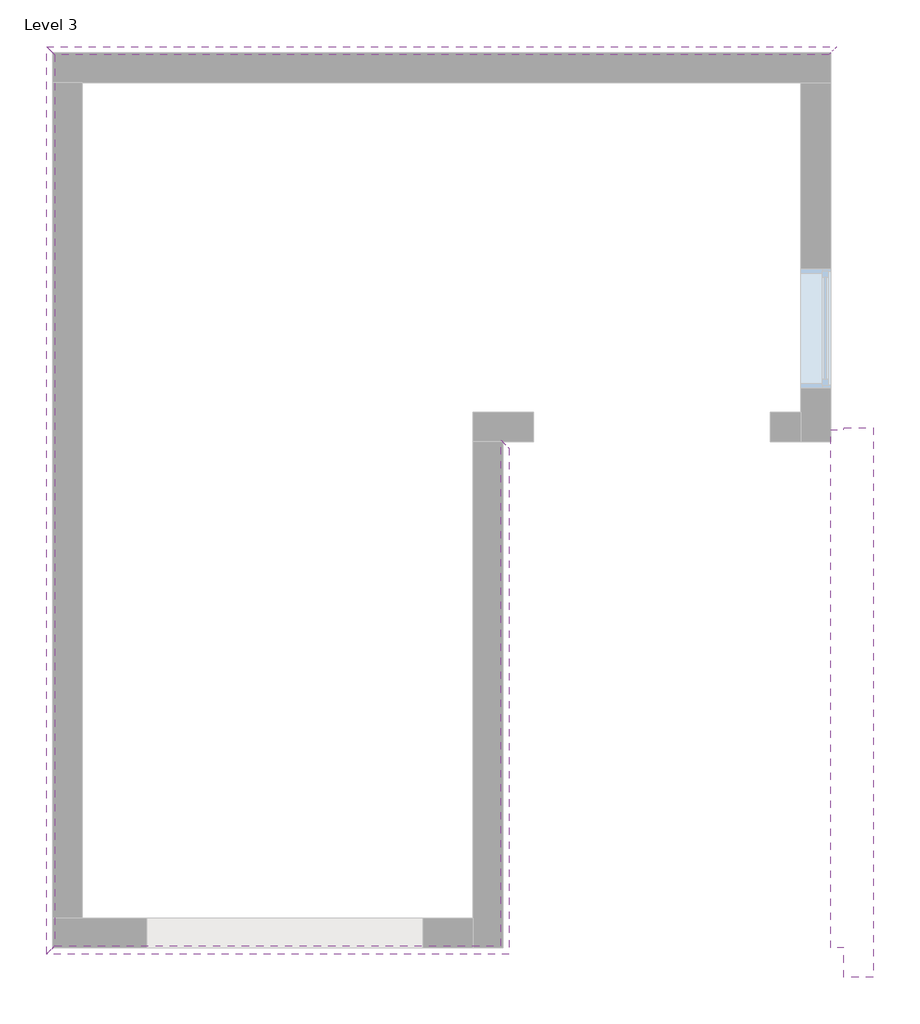
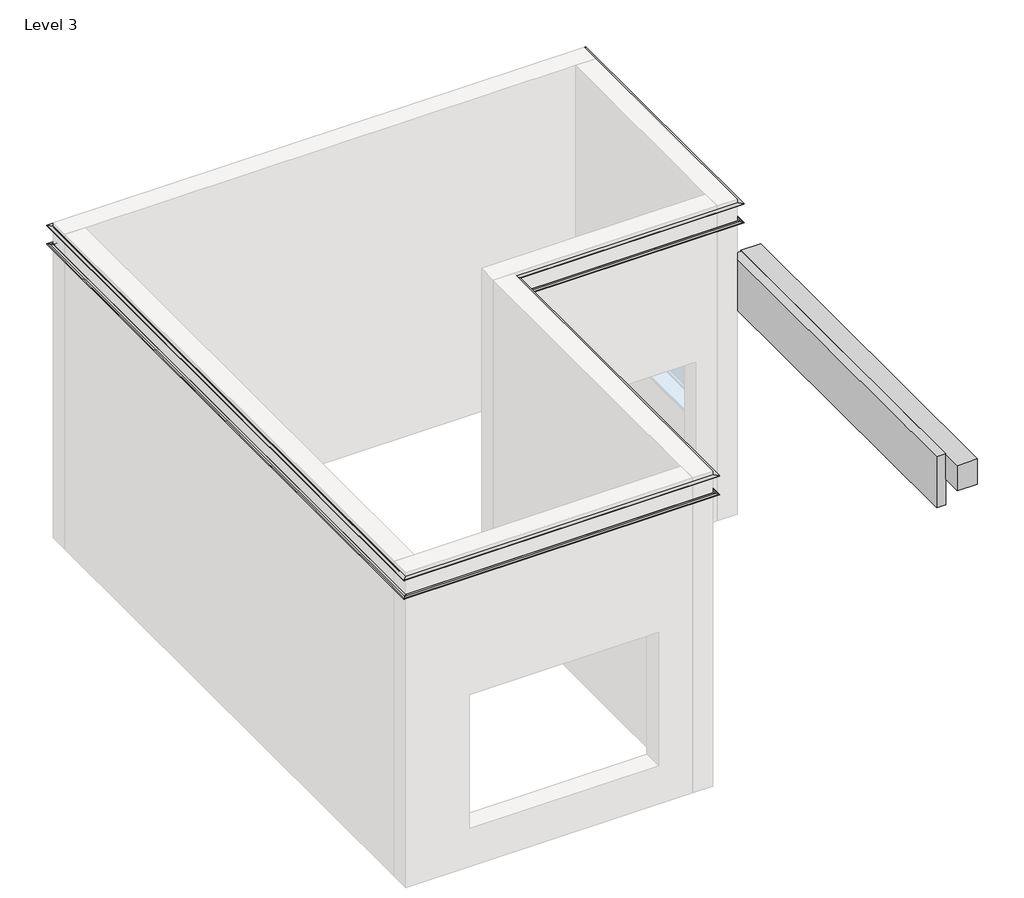
# One storey, part 2 of 2: 4 proxies.
"""IFC4 building model written with IfcOpenShell, lengths in millimetres."""

from ifc_helpers import new_model, si_unit, frame, origin, place, context, project, spatial, polyline, ellipse_curve, transform, mapped, element, save
from ifc_brep_helpers import plane_surface, cylinder_surface, revolved_surface, advanced_brep
from components import generic_models_3_generic_models_3_e8135b9d

model = new_model("IFC4")

# Units and contexts
model_context = context("Model", 3, world=origin())
ifc_project = project(units=[si_unit("LENGTHUNIT", "METRE", prefix="MILLI")], contexts=[model_context])

# Site, building, storey
site = spatial("IfcSite", under=ifc_project)
building = spatial("IfcBuilding", under=site)
storey = spatial("IfcBuildingStorey", under=building, Name="Level 3", Elevation=3200.4)

# Proxies
placement = place(None, origin())
element("IfcBuildingElementProxy", 1, Name="Cornice", ObjectType="Cornice", at=placement, inside=storey, context=model_context, shape_type="AdvancedBrep", body=[
    advanced_brep(
    [(-9818.4141584, 755.0106137, 6921.5), (-9755.1681584, 691.7646137, 6921.5), (-9755.1681584, 691.7646137, 6920.1203242), (-9759.5509676, 696.1474229, 6914.9465897), (-9783.1716584, 719.7681137, 6911.0098), (-9802.40954, 739.0059953, 6907.80348), (-9811.1751584, 747.7716137, 6897.456011), (-9811.1751584, 747.7716137, 6716.943989), (-9802.40954, 739.0059953, 6706.59652), (-9783.1716584, 719.7681137, 6703.3902), (-9759.5509676, 696.1474229, 6699.4534103), (-9755.1681584, 691.7646137, 6694.2796758), (-9755.1681584, 691.7646137, 6692.9), (-9818.4141584, 755.0106137, 6692.9), (-13260.1109834, 755.0106137, 6921.5), (-13260.1109834, 755.0106137, 6692.9), (-13323.3569834, 691.7646137, 6692.9), (-13323.3569834, 691.7646137, 6694.2796758), (-13318.9741742, 696.1474229, 6699.4534103), (-13295.3534834, 719.7681137, 6703.3902), (-13276.1156018, 739.0059953, 6706.59652), (-13267.3499834, 747.7716137, 6716.943989), (-13267.3499834, 747.7716137, 6897.456011), (-13276.1156018, 739.0059953, 6907.80348), (-13295.3534834, 719.7681137, 6911.0098), (-13318.9741742, 696.1474229, 6914.9465897), (-13323.3569834, 691.7646137, 6920.1203242), (-13323.3569834, 691.7646137, 6921.5)],
    [
        (0, 1),
        (1, 2),
        (2, 3, ellipse_curve(frame((-9760.4132584, 697.0097137, 6920.1203242), z_axis=(0.7071067811865493, 0.7071067811865458, 0.0), x_axis=(0.7071067811865456, -0.7071067811865493, 0.0)), 7.4176916, 5.2451)),
        (3, 4),
        (4, 5),
        (5, 6, ellipse_curve(frame((-9800.6849584, 737.2814137, 6897.456011), z_axis=(-0.7071067811865493, -0.7071067811865458, 0.0), x_axis=(-0.7071067811865456, 0.7071067811865493, 0.0)), 14.8353831, 10.4902)),
        (6, 7),
        (7, 8, ellipse_curve(frame((-9800.6849584, 737.2814137, 6716.943989), z_axis=(-0.7071067811865493, -0.7071067811865458, 0.0), x_axis=(-0.7071067811865456, 0.7071067811865493, 0.0)), 14.8353831, 10.4902)),
        (8, 9),
        (9, 10),
        (10, 11, ellipse_curve(frame((-9760.4132584, 697.0097137, 6694.2796758), z_axis=(0.7071067811865493, 0.7071067811865458, 0.0), x_axis=(0.7071067811865456, -0.7071067811865493, 0.0)), 7.4176916, 5.2451)),
        (11, 12),
        (12, 13),
        (13, 0),
        (14, 15),
        (15, 16),
        (16, 17),
        (17, 18, ellipse_curve(frame((-13318.1118834, 697.0097137, 6694.2796758), z_axis=(-0.7071067811865436, 0.7071067811865516, 0.0), x_axis=(0.7071067811865515, 0.7071067811865437, 0.0)), 7.4176916, 5.2451)),
        (18, 19),
        (19, 20),
        (20, 21, ellipse_curve(frame((-13277.8401834, 737.2814137, 6716.943989), z_axis=(0.7071067811865436, -0.7071067811865516, 0.0), x_axis=(-0.7071067811865515, -0.7071067811865437, 0.0)), 14.8353831, 10.4902)),
        (21, 22),
        (22, 23, ellipse_curve(frame((-13277.8401834, 737.2814137, 6897.456011), z_axis=(0.7071067811865436, -0.7071067811865516, 0.0), x_axis=(-0.7071067811865515, -0.7071067811865437, 0.0)), 14.8353831, 10.4902)),
        (23, 24),
        (24, 25),
        (25, 26, ellipse_curve(frame((-13318.1118834, 697.0097137, 6920.1203242), z_axis=(-0.7071067811865436, 0.7071067811865516, 0.0), x_axis=(0.7071067811865515, 0.7071067811865437, 0.0)), 7.4176916, 5.2451)),
        (26, 27),
        (27, 14),
        (0, 14),
        (27, 1),
        (26, 2),
        (25, 3),
        (24, 4),
        (23, 5),
        (22, 6),
        (21, 7),
        (20, 8),
        (19, 9),
        (18, 10),
        (17, 11),
        (16, 12),
        (15, 13),
    ],
    [
        plane_surface(frame((-9803.5297584, 740.1262137, 7112.0), z_axis=(0.7071067811865493, 0.7071067811865458, 0.0), x_axis=(-0.7071067811865458, 0.7071067811865493, 0.0))),
        plane_surface(frame((-13274.9953834, 740.1262137, 7112.0), z_axis=(-0.7071067811865436, 0.7071067811865516, 0.0), x_axis=(0.7071067811865516, 0.7071067811865436, 0.0))),
        plane_surface(frame((-9818.4141584, 755.0106137, 6921.5), z_axis=(0.0, 0.0, 1.0), x_axis=(-1.0, 0.0, 0.0))),
        plane_surface(frame((-9755.1681584, 691.7646137, 6921.5), z_axis=(0.0, -1.0, 0.0), x_axis=(-1.0, 0.0, 0.0))),
        cylinder_surface(frame((-9803.5297584, 697.0097137, 6920.1203242), z_axis=(1.0, 0.0, 0.0), x_axis=(0.0, -1.0, 0.0)), 5.2451),
        plane_surface(frame((-9759.5509676, 696.1474229, 6914.9465897), z_axis=(0.0, -0.16439930721687082, -0.9863938705135049), x_axis=(-1.0, 0.0, 0.0))),
        plane_surface(frame((-9783.1716584, 719.7681137, 6911.0098), z_axis=(0.0, -0.16439930721687146, -0.9863938705135048), x_axis=(-1.0, 0.0, 0.0))),
        revolved_surface(polyline([(-13288.33038339151, 726.7912137000001, 6897.456011), (-9790.194758408488, 726.7912137000001, 6897.456011)]), (-9803.5297584, 737.2814137, 6897.456011), (-1.0, 0.0, 0.0)),
        plane_surface(frame((-9811.1751584, 747.7716137, 6897.456011), z_axis=(0.0, -1.0, 0.0), x_axis=(-1.0, 0.0, 0.0))),
        revolved_surface(polyline([(-13288.33038339151, 726.7912137000001, 6716.943989), (-9790.194758408488, 726.7912137000001, 6716.943989)]), (-9803.5297584, 737.2814137, 6716.943989), (-1.0, 0.0, 0.0)),
        plane_surface(frame((-9802.40954, 739.0059953, 6706.59652), z_axis=(0.0, -0.1643993072168769, 0.9863938705135039), x_axis=(-1.0, 0.0, 0.0))),
        plane_surface(frame((-9783.1716584, 719.7681137, 6703.3902), z_axis=(0.0, -0.16439930721687793, 0.9863938705135037), x_axis=(-1.0, 0.0, 0.0))),
        cylinder_surface(frame((-9803.5297584, 697.0097137, 6694.2796758), z_axis=(1.0, 0.0, 0.0), x_axis=(0.0, -1.0, 0.0)), 5.2451),
        plane_surface(frame((-9755.1681584, 691.7646137, 6694.2796758), z_axis=(0.0, -1.0, 0.0), x_axis=(-1.0, 0.0, 0.0))),
        plane_surface(frame((-9755.1681584, 691.7646137, 6692.9), z_axis=(0.0, 0.0, -1.0), x_axis=(-1.0, 0.0, 0.0))),
        plane_surface(frame((-9818.4141584, 755.0106137, 6692.9), z_axis=(0.0, 1.0, 0.0), x_axis=(-1.0, 0.0, 0.0))),
    ],
    [
        (0, [[1, 2, 3, 4, 5, 6, 7, 8, 9, 10, 11, 12, 13, 14]]),
        (1, [[15, 16, 17, 18, 19, 20, 21, 22, 23, 24, 25, 26, 27, 28]]),
        (2, [[-1, 29, -28, 30]]),
        (3, [[-2, -30, -27, 31]]),
        (4, [[-3, -31, -26, 32]]),
        (5, [[-4, -32, -25, 33]]),
        (6, [[-5, -33, -24, 34]]),
        (7, [[-6, -34, -23, 35]]),
        (8, [[-7, -35, -22, 36]]),
        (9, [[-8, -36, -21, 37]]),
        (10, [[-9, -37, -20, 38]]),
        (11, [[-10, -38, -19, 39]]),
        (12, [[-11, -39, -18, 40]]),
        (13, [[-12, -40, -17, 41]]),
        (14, [[-13, -41, -16, 42]]),
        (15, [[-14, -42, -15, -29]]),
    ],
),
    advanced_brep(
    [(-9818.4141584, 4655.0020199, 6921.5), (-9755.1681584, 4591.7560199, 6921.5), (-9755.1681584, 4591.7560199, 6920.1203242), (-9759.5509676, 4596.1388291, 6914.9465897), (-9783.1716584, 4619.7595199, 6911.0098), (-9802.40954, 4638.9974015, 6907.80348), (-9811.1751584, 4647.7630199, 6897.456011), (-9811.1751584, 4647.7630199, 6716.943989), (-9802.40954, 4638.9974015, 6706.59652), (-9783.1716584, 4619.7595199, 6703.3902), (-9759.5509676, 4596.1388291, 6699.4534103), (-9755.1681584, 4591.7560199, 6694.2796758), (-9755.1681584, 4591.7560199, 6692.9), (-9818.4141584, 4655.0020199, 6692.9), (-9818.4141584, 755.0106137, 6921.5), (-9818.4141584, 755.0106137, 6692.9), (-9755.1681584, 691.7646137, 6692.9), (-9755.1681584, 691.7646137, 6694.2796758), (-9759.5509676, 696.1474229, 6699.4534103), (-9783.1716584, 719.7681137, 6703.3902), (-9802.40954, 739.0059953, 6706.59652), (-9811.1751584, 747.7716137, 6716.943989), (-9811.1751584, 747.7716137, 6897.456011), (-9802.40954, 739.0059953, 6907.80348), (-9783.1716584, 719.7681137, 6911.0098), (-9759.5509676, 696.1474229, 6914.9465897), (-9755.1681584, 691.7646137, 6920.1203242), (-9755.1681584, 691.7646137, 6921.5)],
    [
        (0, 1),
        (1, 2),
        (2, 3, ellipse_curve(frame((-9760.4132584, 4597.0011199, 6920.1203242), z_axis=(0.7071067811865493, 0.7071067811865458, 0.0), x_axis=(-0.7071067811865458, 0.7071067811865492, 0.0)), 7.4176916, 5.2451)),
        (3, 4),
        (4, 5),
        (5, 6, ellipse_curve(frame((-9800.6849584, 4637.2728199, 6897.456011), z_axis=(-0.7071067811865493, -0.7071067811865458, 0.0), x_axis=(0.7071067811865458, -0.7071067811865492, 0.0)), 14.8353831, 10.4902)),
        (6, 7),
        (7, 8, ellipse_curve(frame((-9800.6849584, 4637.2728199, 6716.943989), z_axis=(-0.7071067811865493, -0.7071067811865458, 0.0), x_axis=(0.7071067811865458, -0.7071067811865492, 0.0)), 14.8353831, 10.4902)),
        (8, 9),
        (9, 10),
        (10, 11, ellipse_curve(frame((-9760.4132584, 4597.0011199, 6694.2796758), z_axis=(0.7071067811865493, 0.7071067811865458, 0.0), x_axis=(-0.7071067811865458, 0.7071067811865492, 0.0)), 7.4176916, 5.2451)),
        (11, 12),
        (12, 13),
        (13, 0),
        (14, 15),
        (15, 16),
        (16, 17),
        (17, 18, ellipse_curve(frame((-9760.4132584, 697.0097137, 6694.2796758), z_axis=(-0.7071067811865493, -0.7071067811865458, 0.0), x_axis=(-0.7071067811865458, 0.7071067811865492, 0.0)), 7.4176916, 5.2451)),
        (18, 19),
        (19, 20),
        (20, 21, ellipse_curve(frame((-9800.6849584, 737.2814137, 6716.943989), z_axis=(0.7071067811865493, 0.7071067811865458, 0.0), x_axis=(0.7071067811865458, -0.7071067811865492, 0.0)), 14.8353831, 10.4902)),
        (21, 22),
        (22, 23, ellipse_curve(frame((-9800.6849584, 737.2814137, 6897.456011), z_axis=(0.7071067811865493, 0.7071067811865458, 0.0), x_axis=(0.7071067811865458, -0.7071067811865492, 0.0)), 14.8353831, 10.4902)),
        (23, 24),
        (24, 25),
        (25, 26, ellipse_curve(frame((-9760.4132584, 697.0097137, 6920.1203242), z_axis=(-0.7071067811865493, -0.7071067811865458, 0.0), x_axis=(-0.7071067811865458, 0.7071067811865492, 0.0)), 7.4176916, 5.2451)),
        (26, 27),
        (27, 14),
        (0, 14),
        (27, 1),
        (26, 2),
        (25, 3),
        (24, 4),
        (23, 5),
        (22, 6),
        (21, 7),
        (20, 8),
        (19, 9),
        (18, 10),
        (17, 11),
        (16, 12),
        (15, 13),
    ],
    [
        plane_surface(frame((-9803.5297584, 4640.1176199, 6502.4), z_axis=(0.7071067811865493, 0.7071067811865458, 0.0), x_axis=(0.7071067811865458, -0.7071067811865493, 0.0))),
        plane_surface(frame((-9803.5297584, 740.1262137, 7112.0), z_axis=(-0.7071067811865493, -0.7071067811865458, 0.0), x_axis=(-0.7071067811865458, 0.7071067811865493, 0.0))),
        plane_surface(frame((-9818.4141584, 4655.0020199, 6921.5), z_axis=(0.0, 0.0, 1.0), x_axis=(0.0, -1.0, 0.0))),
        plane_surface(frame((-9755.1681584, 4591.7560199, 6921.5), z_axis=(1.0, 0.0, 0.0), x_axis=(0.0, -1.0, 0.0))),
        cylinder_surface(frame((-9760.4132584, 4640.1176199, 6920.1203242), z_axis=(0.0, 1.0, 0.0), x_axis=(1.0, 0.0, 0.0)), 5.2451),
        plane_surface(frame((-9759.5509676, 4596.1388291, 6914.9465897), z_axis=(0.16439930721687082, 0.0, -0.9863938705135049), x_axis=(0.0, -1.0, 0.0))),
        plane_surface(frame((-9783.1716584, 4619.7595199, 6911.0098), z_axis=(0.16439930721687146, 0.0, -0.9863938705135048), x_axis=(0.0, -1.0, 0.0))),
        revolved_surface(polyline([(-9790.194758399999, 726.7912137084895, 6897.456011), (-9790.194758399999, 4647.7630199, 6897.456011)]), (-9800.6849584, 4640.1176199, 6897.456011), (0.0, -1.0, 0.0)),
        plane_surface(frame((-9811.1751584, 4647.7630199, 6897.456011), z_axis=(1.0, 0.0, 0.0), x_axis=(0.0, -1.0, 0.0))),
        revolved_surface(polyline([(-9790.194758399999, 726.7912137084895, 6716.943989), (-9790.194758399999, 4647.7630199, 6716.943989)]), (-9800.6849584, 4640.1176199, 6716.943989), (0.0, -1.0, 0.0)),
        plane_surface(frame((-9802.40954, 4638.9974015, 6706.59652), z_axis=(0.1643993072168769, 0.0, 0.9863938705135039), x_axis=(0.0, -1.0, 0.0))),
        plane_surface(frame((-9783.1716584, 4619.7595199, 6703.3902), z_axis=(0.16439930721687793, 0.0, 0.9863938705135037), x_axis=(0.0, -1.0, 0.0))),
        cylinder_surface(frame((-9760.4132584, 4640.1176199, 6694.2796758), z_axis=(0.0, 1.0, 0.0), x_axis=(1.0, 0.0, 0.0)), 5.2451),
        plane_surface(frame((-9755.1681584, 4591.7560199, 6694.2796758), z_axis=(1.0, 0.0, 0.0), x_axis=(0.0, -1.0, 0.0))),
        plane_surface(frame((-9755.1681584, 4591.7560199, 6692.9), z_axis=(0.0, 0.0, -1.0), x_axis=(0.0, -1.0, 0.0))),
        plane_surface(frame((-9818.4141584, 4655.0020199, 6692.9), z_axis=(-1.0, 0.0, 0.0), x_axis=(0.0, -1.0, 0.0))),
    ],
    [
        (0, [[1, 2, 3, 4, 5, 6, 7, 8, 9, 10, 11, 12, 13, 14]]),
        (1, [[15, 16, 17, 18, 19, 20, 21, 22, 23, 24, 25, 26, 27, 28]]),
        (2, [[-1, 29, -28, 30]]),
        (3, [[-2, -30, -27, 31]]),
        (4, [[-3, -31, -26, 32]]),
        (5, [[-4, -32, -25, 33]]),
        (6, [[-5, -33, -24, 34]]),
        (7, [[-6, -34, -23, 35]]),
        (8, [[-7, -35, -22, 36]]),
        (9, [[-8, -36, -21, 37]]),
        (10, [[-9, -37, -20, 38]]),
        (11, [[-10, -38, -19, 39]]),
        (12, [[-11, -39, -18, 40]]),
        (13, [[-12, -40, -17, 41]]),
        (14, [[-13, -41, -16, 42]]),
        (15, [[-14, -42, -15, -29]]),
    ],
),
])
element("IfcBuildingElementProxy", 2, Name="Cornice", ObjectType="Cornice", at=placement, inside=storey, context=model_context, shape_type="AdvancedBrep", body=[
    advanced_brep(
    [(-7289.8797834, 4655.0020199, 6921.5), (-7226.6337834, 4591.7560199, 6921.5), (-7226.6337834, 4591.7560199, 6920.1203242), (-7231.0165926, 4596.1388291, 6914.9465897), (-7254.6372834, 4619.7595199, 6911.0098), (-7273.875165, 4638.9974015, 6907.80348), (-7282.6407834, 4647.7630199, 6897.456011), (-7282.6407834, 4647.7630199, 6716.943989), (-7273.875165, 4638.9974015, 6706.59652), (-7254.6372834, 4619.7595199, 6703.3902), (-7231.0165926, 4596.1388291, 6699.4534103), (-7226.6337834, 4591.7560199, 6694.2796758), (-7226.6337834, 4591.7560199, 6692.9), (-7289.8797834, 4655.0020199, 6692.9), (-9818.4141584, 4655.0020199, 6921.5), (-9818.4141584, 4655.0020199, 6692.9), (-9755.1681584, 4591.7560199, 6692.9), (-9755.1681584, 4591.7560199, 6694.2796758), (-9759.5509676, 4596.1388291, 6699.4534103), (-9783.1716584, 4619.7595199, 6703.3902), (-9802.40954, 4638.9974015, 6706.59652), (-9811.1751584, 4647.7630199, 6716.943989), (-9811.1751584, 4647.7630199, 6897.456011), (-9802.40954, 4638.9974015, 6907.80348), (-9783.1716584, 4619.7595199, 6911.0098), (-9759.5509676, 4596.1388291, 6914.9465897), (-9755.1681584, 4591.7560199, 6920.1203242), (-9755.1681584, 4591.7560199, 6921.5)],
    [
        (0, 1),
        (1, 2),
        (2, 3, ellipse_curve(frame((-7231.8788834, 4597.0011199, 6920.1203242), z_axis=(0.707106781186552, 0.7071067811865431, 0.0), x_axis=(0.7071067811865431, -0.707106781186552, 0.0)), 7.4176916, 5.2451)),
        (3, 4),
        (4, 5),
        (5, 6, ellipse_curve(frame((-7272.1505834, 4637.2728199, 6897.456011), z_axis=(-0.707106781186552, -0.7071067811865431, 0.0), x_axis=(-0.7071067811865431, 0.707106781186552, 0.0)), 14.8353831, 10.4902)),
        (6, 7),
        (7, 8, ellipse_curve(frame((-7272.1505834, 4637.2728199, 6716.943989), z_axis=(-0.707106781186552, -0.7071067811865431, 0.0), x_axis=(-0.7071067811865431, 0.707106781186552, 0.0)), 14.8353831, 10.4902)),
        (8, 9),
        (9, 10),
        (10, 11, ellipse_curve(frame((-7231.8788834, 4597.0011199, 6694.2796758), z_axis=(0.707106781186552, 0.7071067811865431, 0.0), x_axis=(0.7071067811865431, -0.707106781186552, 0.0)), 7.4176916, 5.2451)),
        (11, 12),
        (12, 13),
        (13, 0),
        (14, 15),
        (15, 16),
        (16, 17),
        (17, 18, ellipse_curve(frame((-9760.4132584, 4597.0011199, 6694.2796758), z_axis=(-0.7071067811865493, -0.7071067811865458, 0.0), x_axis=(0.7071067811865458, -0.7071067811865493, 0.0)), 7.4176916, 5.2451)),
        (18, 19),
        (19, 20),
        (20, 21, ellipse_curve(frame((-9800.6849584, 4637.2728199, 6716.943989), z_axis=(0.7071067811865493, 0.7071067811865458, 0.0), x_axis=(-0.7071067811865458, 0.7071067811865493, 0.0)), 14.8353831, 10.4902)),
        (21, 22),
        (22, 23, ellipse_curve(frame((-9800.6849584, 4637.2728199, 6897.456011), z_axis=(0.7071067811865493, 0.7071067811865458, 0.0), x_axis=(-0.7071067811865458, 0.7071067811865493, 0.0)), 14.8353831, 10.4902)),
        (23, 24),
        (24, 25),
        (25, 26, ellipse_curve(frame((-9760.4132584, 4597.0011199, 6920.1203242), z_axis=(-0.7071067811865493, -0.7071067811865458, 0.0), x_axis=(0.7071067811865458, -0.7071067811865493, 0.0)), 7.4176916, 5.2451)),
        (26, 27),
        (27, 14),
        (0, 14),
        (27, 1),
        (26, 2),
        (25, 3),
        (24, 4),
        (23, 5),
        (22, 6),
        (21, 7),
        (20, 8),
        (19, 9),
        (18, 10),
        (17, 11),
        (16, 12),
        (15, 13),
    ],
    [
        plane_surface(frame((-7274.9953834, 4640.1176199, 7112.0), z_axis=(0.707106781186552, 0.7071067811865431, 0.0), x_axis=(-0.7071067811865431, 0.707106781186552, 0.0))),
        plane_surface(frame((-9803.5297584, 4640.1176199, 6502.4), z_axis=(-0.7071067811865493, -0.7071067811865458, 0.0), x_axis=(0.7071067811865458, -0.7071067811865493, 0.0))),
        plane_surface(frame((-7289.8797834, 4655.0020199, 6921.5), z_axis=(0.0, 0.0, 1.0), x_axis=(-1.0, 0.0, 0.0))),
        plane_surface(frame((-7226.6337834, 4591.7560199, 6921.5), z_axis=(0.0, -1.0, 0.0), x_axis=(-1.0, 0.0, 0.0))),
        cylinder_surface(frame((-7274.9953834, 4597.0011199, 6920.1203242), z_axis=(1.0, 0.0, 0.0), x_axis=(0.0, -1.0, 0.0)), 5.2451),
        plane_surface(frame((-7231.0165926, 4596.1388291, 6914.9465897), z_axis=(0.0, -0.16439930721687082, -0.9863938705135049), x_axis=(-1.0, 0.0, 0.0))),
        plane_surface(frame((-7254.6372834, 4619.7595199, 6911.0098), z_axis=(0.0, -0.16439930721687146, -0.9863938705135048), x_axis=(-1.0, 0.0, 0.0))),
        revolved_surface(polyline([(-9811.1751584, 4626.7826199, 6897.456011), (-7261.66038340849, 4626.7826199, 6897.456011)]), (-7274.9953834, 4637.2728199, 6897.456011), (-1.0, 0.0, 0.0)),
        plane_surface(frame((-7282.6407834, 4647.7630199, 6897.456011), z_axis=(0.0, -1.0, 0.0), x_axis=(-1.0, 0.0, 0.0))),
        revolved_surface(polyline([(-9811.1751584, 4626.7826199, 6716.943989), (-7261.66038340849, 4626.7826199, 6716.943989)]), (-7274.9953834, 4637.2728199, 6716.943989), (-1.0, 0.0, 0.0)),
        plane_surface(frame((-7273.875165, 4638.9974015, 6706.59652), z_axis=(0.0, -0.1643993072168769, 0.9863938705135039), x_axis=(-1.0, 0.0, 0.0))),
        plane_surface(frame((-7254.6372834, 4619.7595199, 6703.3902), z_axis=(0.0, -0.16439930721687793, 0.9863938705135037), x_axis=(-1.0, 0.0, 0.0))),
        cylinder_surface(frame((-7274.9953834, 4597.0011199, 6694.2796758), z_axis=(1.0, 0.0, 0.0), x_axis=(0.0, -1.0, 0.0)), 5.2451),
        plane_surface(frame((-7226.6337834, 4591.7560199, 6694.2796758), z_axis=(0.0, -1.0, 0.0), x_axis=(-1.0, 0.0, 0.0))),
        plane_surface(frame((-7226.6337834, 4591.7560199, 6692.9), z_axis=(0.0, 0.0, -1.0), x_axis=(-1.0, 0.0, 0.0))),
        plane_surface(frame((-7289.8797834, 4655.0020199, 6692.9), z_axis=(0.0, 1.0, 0.0), x_axis=(-1.0, 0.0, 0.0))),
    ],
    [
        (0, [[1, 2, 3, 4, 5, 6, 7, 8, 9, 10, 11, 12, 13, 14]]),
        (1, [[15, 16, 17, 18, 19, 20, 21, 22, 23, 24, 25, 26, 27, 28]]),
        (2, [[-1, 29, -28, 30]]),
        (3, [[-2, -30, -27, 31]]),
        (4, [[-3, -31, -26, 32]]),
        (5, [[-4, -32, -25, 33]]),
        (6, [[-5, -33, -24, 34]]),
        (7, [[-6, -34, -23, 35]]),
        (8, [[-7, -35, -22, 36]]),
        (9, [[-8, -36, -21, 37]]),
        (10, [[-9, -37, -20, 38]]),
        (11, [[-10, -38, -19, 39]]),
        (12, [[-11, -39, -18, 40]]),
        (13, [[-12, -40, -17, 41]]),
        (14, [[-13, -41, -16, 42]]),
        (15, [[-14, -42, -15, -29]]),
    ],
),
    advanced_brep(
    [(-7289.8797834, 7625.2418137, 6921.5), (-7226.6337834, 7688.4878137, 6921.5), (-7226.6337834, 7688.4878137, 6920.1203242), (-7231.0165926, 7684.1050045, 6914.9465897), (-7254.6372834, 7660.4843137, 6911.0098), (-7273.875165, 7641.2464321, 6907.80348), (-7282.6407834, 7632.4808137, 6897.456011), (-7282.6407834, 7632.4808137, 6716.943989), (-7273.875165, 7641.2464321, 6706.59652), (-7254.6372834, 7660.4843137, 6703.3902), (-7231.0165926, 7684.1050045, 6699.4534103), (-7226.6337834, 7688.4878137, 6694.2796758), (-7226.6337834, 7688.4878137, 6692.9), (-7289.8797834, 7625.2418137, 6692.9), (-7289.8797834, 4655.0020199, 6921.5), (-7289.8797834, 4655.0020199, 6692.9), (-7226.6337834, 4591.7560199, 6692.9), (-7226.6337834, 4591.7560199, 6694.2796758), (-7231.0165926, 4596.1388291, 6699.4534103), (-7254.6372834, 4619.7595199, 6703.3902), (-7273.875165, 4638.9974015, 6706.59652), (-7282.6407834, 4647.7630199, 6716.943989), (-7282.6407834, 4647.7630199, 6897.456011), (-7273.875165, 4638.9974015, 6907.80348), (-7254.6372834, 4619.7595199, 6911.0098), (-7231.0165926, 4596.1388291, 6914.9465897), (-7226.6337834, 4591.7560199, 6920.1203242), (-7226.6337834, 4591.7560199, 6921.5)],
    [
        (0, 1),
        (1, 2),
        (2, 3, ellipse_curve(frame((-7231.8788834, 7683.2427137, 6920.1203242), z_axis=(-0.7071067811865458, 0.7071067811865493, 0.0), x_axis=(0.7071067811865493, 0.7071067811865456, 0.0)), 7.4176916, 5.2451)),
        (3, 4),
        (4, 5),
        (5, 6, ellipse_curve(frame((-7272.1505834, 7642.9710137, 6897.456011), z_axis=(0.7071067811865458, -0.7071067811865493, 0.0), x_axis=(-0.7071067811865493, -0.7071067811865456, 0.0)), 14.8353831, 10.4902)),
        (6, 7),
        (7, 8, ellipse_curve(frame((-7272.1505834, 7642.9710137, 6716.943989), z_axis=(0.7071067811865458, -0.7071067811865493, 0.0), x_axis=(-0.7071067811865493, -0.7071067811865456, 0.0)), 14.8353831, 10.4902)),
        (8, 9),
        (9, 10),
        (10, 11, ellipse_curve(frame((-7231.8788834, 7683.2427137, 6694.2796758), z_axis=(-0.7071067811865458, 0.7071067811865493, 0.0), x_axis=(0.7071067811865493, 0.7071067811865456, 0.0)), 7.4176916, 5.2451)),
        (11, 12),
        (12, 13),
        (13, 0),
        (14, 15),
        (15, 16),
        (16, 17),
        (17, 18, ellipse_curve(frame((-7231.8788834, 4597.0011199, 6694.2796758), z_axis=(-0.707106781186552, -0.7071067811865431, 0.0), x_axis=(-0.7071067811865432, 0.7071067811865518, 0.0)), 7.4176916, 5.2451)),
        (18, 19),
        (19, 20),
        (20, 21, ellipse_curve(frame((-7272.1505834, 4637.2728199, 6716.943989), z_axis=(0.707106781186552, 0.7071067811865431, 0.0), x_axis=(0.7071067811865432, -0.7071067811865518, 0.0)), 14.8353831, 10.4902)),
        (21, 22),
        (22, 23, ellipse_curve(frame((-7272.1505834, 4637.2728199, 6897.456011), z_axis=(0.707106781186552, 0.7071067811865431, 0.0), x_axis=(0.7071067811865432, -0.7071067811865518, 0.0)), 14.8353831, 10.4902)),
        (23, 24),
        (24, 25),
        (25, 26, ellipse_curve(frame((-7231.8788834, 4597.0011199, 6920.1203242), z_axis=(-0.707106781186552, -0.7071067811865431, 0.0), x_axis=(-0.7071067811865432, 0.7071067811865518, 0.0)), 7.4176916, 5.2451)),
        (26, 27),
        (27, 14),
        (0, 14),
        (27, 1),
        (26, 2),
        (25, 3),
        (24, 4),
        (23, 5),
        (22, 6),
        (21, 7),
        (20, 8),
        (19, 9),
        (18, 10),
        (17, 11),
        (16, 12),
        (15, 13),
    ],
    [
        plane_surface(frame((-7274.9953834, 7640.1262137, 7112.0), z_axis=(-0.7071067811865458, 0.7071067811865493, 0.0), x_axis=(-0.7071067811865493, -0.7071067811865458, 0.0))),
        plane_surface(frame((-7274.9953834, 4640.1176199, 7112.0), z_axis=(-0.707106781186552, -0.7071067811865431, 0.0), x_axis=(-0.7071067811865431, 0.707106781186552, 0.0))),
        plane_surface(frame((-7289.8797834, 7625.2418137, 6921.5), z_axis=(0.0, 0.0, 1.0), x_axis=(0.0, -1.0, 0.0))),
        plane_surface(frame((-7226.6337834, 7688.4878137, 6921.5), z_axis=(1.0, 0.0, 0.0), x_axis=(0.0, -1.0, 0.0))),
        cylinder_surface(frame((-7231.8788834, 7640.1262137, 6920.1203242), z_axis=(0.0, 1.0, 0.0), x_axis=(1.0, 0.0, 0.0)), 5.2451),
        plane_surface(frame((-7231.0165926, 7684.1050045, 6914.9465897), z_axis=(0.16439930721687082, 0.0, -0.9863938705135049), x_axis=(0.0, -1.0, 0.0))),
        plane_surface(frame((-7254.6372834, 7660.4843137, 6911.0098), z_axis=(0.16439930721687146, 0.0, -0.9863938705135048), x_axis=(0.0, -1.0, 0.0))),
        revolved_surface(polyline([(-7261.6603834, 4626.78261990849, 6897.456011), (-7261.6603834, 7653.46121369151, 6897.456011)]), (-7272.1505834, 7640.1262137, 6897.456011), (0.0, -1.0, 0.0)),
        plane_surface(frame((-7282.6407834, 7632.4808137, 6897.456011), z_axis=(1.0, 0.0, 0.0), x_axis=(0.0, -1.0, 0.0))),
        revolved_surface(polyline([(-7261.6603834, 4626.78261990849, 6716.943989), (-7261.6603834, 7653.46121369151, 6716.943989)]), (-7272.1505834, 7640.1262137, 6716.943989), (0.0, -1.0, 0.0)),
        plane_surface(frame((-7273.875165, 7641.2464321, 6706.59652), z_axis=(0.1643993072168769, 0.0, 0.9863938705135039), x_axis=(0.0, -1.0, 0.0))),
        plane_surface(frame((-7254.6372834, 7660.4843137, 6703.3902), z_axis=(0.16439930721687793, 0.0, 0.9863938705135037), x_axis=(0.0, -1.0, 0.0))),
        cylinder_surface(frame((-7231.8788834, 7640.1262137, 6694.2796758), z_axis=(0.0, 1.0, 0.0), x_axis=(1.0, 0.0, 0.0)), 5.2451),
        plane_surface(frame((-7226.6337834, 7688.4878137, 6694.2796758), z_axis=(1.0, 0.0, 0.0), x_axis=(0.0, -1.0, 0.0))),
        plane_surface(frame((-7226.6337834, 7688.4878137, 6692.9), z_axis=(0.0, 0.0, -1.0), x_axis=(0.0, -1.0, 0.0))),
        plane_surface(frame((-7289.8797834, 7625.2418137, 6692.9), z_axis=(-1.0, 0.0, 0.0), x_axis=(0.0, -1.0, 0.0))),
    ],
    [
        (0, [[1, 2, 3, 4, 5, 6, 7, 8, 9, 10, 11, 12, 13, 14]]),
        (1, [[15, 16, 17, 18, 19, 20, 21, 22, 23, 24, 25, 26, 27, 28]]),
        (2, [[-1, 29, -28, 30]]),
        (3, [[-2, -30, -27, 31]]),
        (4, [[-3, -31, -26, 32]]),
        (5, [[-4, -32, -25, 33]]),
        (6, [[-5, -33, -24, 34]]),
        (7, [[-6, -34, -23, 35]]),
        (8, [[-7, -35, -22, 36]]),
        (9, [[-8, -36, -21, 37]]),
        (10, [[-9, -37, -20, 38]]),
        (11, [[-10, -38, -19, 39]]),
        (12, [[-11, -39, -18, 40]]),
        (13, [[-12, -40, -17, 41]]),
        (14, [[-13, -41, -16, 42]]),
        (15, [[-14, -42, -15, -29]]),
    ],
),
    advanced_brep(
    [(-13260.1109834, 755.0106137, 6921.5), (-13323.3569834, 691.7646137, 6921.5), (-13323.3569834, 691.7646137, 6920.1203242), (-13318.9741742, 696.1474229, 6914.9465897), (-13295.3534834, 719.7681137, 6911.0098), (-13276.1156018, 739.0059953, 6907.80348), (-13267.3499834, 747.7716137, 6897.456011), (-13267.3499834, 747.7716137, 6716.943989), (-13276.1156018, 739.0059953, 6706.59652), (-13295.3534834, 719.7681137, 6703.3902), (-13318.9741742, 696.1474229, 6699.4534103), (-13323.3569834, 691.7646137, 6694.2796758), (-13323.3569834, 691.7646137, 6692.9), (-13260.1109834, 755.0106137, 6692.9), (-13260.1109834, 7625.2418137, 6921.5), (-13260.1109834, 7625.2418137, 6692.9), (-13323.3569834, 7688.4878137, 6692.9), (-13323.3569834, 7688.4878137, 6694.2796758), (-13318.9741742, 7684.1050045, 6699.4534103), (-13295.3534834, 7660.4843137, 6703.3902), (-13276.1156018, 7641.2464321, 6706.59652), (-13267.3499834, 7632.4808137, 6716.943989), (-13267.3499834, 7632.4808137, 6897.456011), (-13276.1156018, 7641.2464321, 6907.80348), (-13295.3534834, 7660.4843137, 6911.0098), (-13318.9741742, 7684.1050045, 6914.9465897), (-13323.3569834, 7688.4878137, 6920.1203242), (-13323.3569834, 7688.4878137, 6921.5)],
    [
        (0, 1),
        (1, 2),
        (2, 3, ellipse_curve(frame((-13318.1118834, 697.0097137, 6920.1203242), z_axis=(0.7071067811865436, -0.7071067811865516, 0.0), x_axis=(-0.7071067811865516, -0.7071067811865435, 0.0)), 7.4176916, 5.2451)),
        (3, 4),
        (4, 5),
        (5, 6, ellipse_curve(frame((-13277.8401834, 737.2814137, 6897.456011), z_axis=(-0.7071067811865436, 0.7071067811865516, 0.0), x_axis=(0.7071067811865516, 0.7071067811865435, 0.0)), 14.8353831, 10.4902)),
        (6, 7),
        (7, 8, ellipse_curve(frame((-13277.8401834, 737.2814137, 6716.943989), z_axis=(-0.7071067811865436, 0.7071067811865516, 0.0), x_axis=(0.7071067811865516, 0.7071067811865435, 0.0)), 14.8353831, 10.4902)),
        (8, 9),
        (9, 10),
        (10, 11, ellipse_curve(frame((-13318.1118834, 697.0097137, 6694.2796758), z_axis=(0.7071067811865436, -0.7071067811865516, 0.0), x_axis=(-0.7071067811865516, -0.7071067811865435, 0.0)), 7.4176916, 5.2451)),
        (11, 12),
        (12, 13),
        (13, 0),
        (14, 15),
        (15, 16),
        (16, 17),
        (17, 18, ellipse_curve(frame((-13318.1118834, 7683.2427137, 6694.2796758), z_axis=(0.7071067811865493, 0.7071067811865458, 0.0), x_axis=(0.7071067811865459, -0.7071067811865492, 0.0)), 7.4176916, 5.2451)),
        (18, 19),
        (19, 20),
        (20, 21, ellipse_curve(frame((-13277.8401834, 7642.9710137, 6716.943989), z_axis=(-0.7071067811865493, -0.7071067811865458, 0.0), x_axis=(-0.7071067811865459, 0.7071067811865492, 0.0)), 14.8353831, 10.4902)),
        (21, 22),
        (22, 23, ellipse_curve(frame((-13277.8401834, 7642.9710137, 6897.456011), z_axis=(-0.7071067811865493, -0.7071067811865458, 0.0), x_axis=(-0.7071067811865459, 0.7071067811865492, 0.0)), 14.8353831, 10.4902)),
        (23, 24),
        (24, 25),
        (25, 26, ellipse_curve(frame((-13318.1118834, 7683.2427137, 6920.1203242), z_axis=(0.7071067811865493, 0.7071067811865458, 0.0), x_axis=(0.7071067811865459, -0.7071067811865492, 0.0)), 7.4176916, 5.2451)),
        (26, 27),
        (27, 14),
        (0, 14),
        (27, 1),
        (26, 2),
        (25, 3),
        (24, 4),
        (23, 5),
        (22, 6),
        (21, 7),
        (20, 8),
        (19, 9),
        (18, 10),
        (17, 11),
        (16, 12),
        (15, 13),
    ],
    [
        plane_surface(frame((-13274.9953834, 740.1262137, 7112.0), z_axis=(0.7071067811865436, -0.7071067811865516, 0.0), x_axis=(0.7071067811865516, 0.7071067811865436, 0.0))),
        plane_surface(frame((-13274.9953834, 7640.1262137, 7112.0), z_axis=(0.7071067811865493, 0.7071067811865458, 0.0), x_axis=(0.7071067811865458, -0.7071067811865493, 0.0))),
        plane_surface(frame((-13260.1109834, 755.0106137, 6921.5), z_axis=(0.0, 0.0, 1.0), x_axis=(0.0, 1.0, 0.0))),
        plane_surface(frame((-13323.3569834, 691.7646137, 6921.5), z_axis=(-1.0, 0.0, 0.0), x_axis=(0.0, 1.0, 0.0))),
        cylinder_surface(frame((-13318.1118834, 740.1262137, 6920.1203242), z_axis=(0.0, -1.0, 0.0), x_axis=(-1.0, 0.0, 0.0)), 5.2451),
        plane_surface(frame((-13318.9741742, 696.1474229, 6914.9465897), z_axis=(-0.16439930721687082, 0.0, -0.9863938705135049), x_axis=(0.0, 1.0, 0.0))),
        plane_surface(frame((-13295.3534834, 719.7681137, 6911.0098), z_axis=(-0.16439930721687146, 0.0, -0.9863938705135048), x_axis=(0.0, 1.0, 0.0))),
        revolved_surface(polyline([(-13288.3303834, 7653.46121369151, 6897.456011), (-13288.3303834, 726.7912137084897, 6897.456011)]), (-13277.8401834, 740.1262137, 6897.456011), (0.0, 1.0, 0.0)),
        plane_surface(frame((-13267.3499834, 747.7716137, 6897.456011), z_axis=(-1.0, 0.0, 0.0), x_axis=(0.0, 1.0, 0.0))),
        revolved_surface(polyline([(-13288.3303834, 7653.46121369151, 6716.943989), (-13288.3303834, 726.7912137084897, 6716.943989)]), (-13277.8401834, 740.1262137, 6716.943989), (0.0, 1.0, 0.0)),
        plane_surface(frame((-13276.1156018, 739.0059953, 6706.59652), z_axis=(-0.1643993072168769, 0.0, 0.9863938705135039), x_axis=(0.0, 1.0, 0.0))),
        plane_surface(frame((-13295.3534834, 719.7681137, 6703.3902), z_axis=(-0.16439930721687793, 0.0, 0.9863938705135037), x_axis=(0.0, 1.0, 0.0))),
        cylinder_surface(frame((-13318.1118834, 740.1262137, 6694.2796758), z_axis=(0.0, -1.0, 0.0), x_axis=(-1.0, 0.0, 0.0)), 5.2451),
        plane_surface(frame((-13323.3569834, 691.7646137, 6694.2796758), z_axis=(-1.0, 0.0, 0.0), x_axis=(0.0, 1.0, 0.0))),
        plane_surface(frame((-13323.3569834, 691.7646137, 6692.9), z_axis=(0.0, 0.0, -1.0), x_axis=(0.0, 1.0, 0.0))),
        plane_surface(frame((-13260.1109834, 755.0106137, 6692.9), z_axis=(1.0, 0.0, 0.0), x_axis=(0.0, 1.0, 0.0))),
    ],
    [
        (0, [[1, 2, 3, 4, 5, 6, 7, 8, 9, 10, 11, 12, 13, 14]]),
        (1, [[15, 16, 17, 18, 19, 20, 21, 22, 23, 24, 25, 26, 27, 28]]),
        (2, [[-1, 29, -28, 30]]),
        (3, [[-2, -30, -27, 31]]),
        (4, [[-3, -31, -26, 32]]),
        (5, [[-4, -32, -25, 33]]),
        (6, [[-5, -33, -24, 34]]),
        (7, [[-6, -34, -23, 35]]),
        (8, [[-7, -35, -22, 36]]),
        (9, [[-8, -36, -21, 37]]),
        (10, [[-9, -37, -20, 38]]),
        (11, [[-10, -38, -19, 39]]),
        (12, [[-11, -39, -18, 40]]),
        (13, [[-12, -40, -17, 41]]),
        (14, [[-13, -41, -16, 42]]),
        (15, [[-14, -42, -15, -29]]),
    ],
),
])
element("IfcBuildingElementProxy", 3, Name="Cornice", ObjectType="Cornice", at=placement, inside=storey, context=model_context, shape_type="AdvancedBrep", body=[
    advanced_brep(
    [(-13260.1109834, 7625.2418137, 6921.5), (-13323.3569834, 7688.4878137, 6921.5), (-13323.3569834, 7688.4878137, 6920.1203242), (-13318.9741742, 7684.1050045, 6914.9465897), (-13295.3534834, 7660.4843137, 6911.0098), (-13276.1156018, 7641.2464321, 6907.80348), (-13267.3499834, 7632.4808137, 6897.456011), (-13267.3499834, 7632.4808137, 6716.943989), (-13276.1156018, 7641.2464321, 6706.59652), (-13295.3534834, 7660.4843137, 6703.3902), (-13318.9741742, 7684.1050045, 6699.4534103), (-13323.3569834, 7688.4878137, 6694.2796758), (-13323.3569834, 7688.4878137, 6692.9), (-13260.1109834, 7625.2418137, 6692.9), (-7289.8797834, 7625.2418137, 6921.5), (-7289.8797834, 7625.2418137, 6692.9), (-7226.6337834, 7688.4878137, 6692.9), (-7226.6337834, 7688.4878137, 6694.2796758), (-7231.0165926, 7684.1050045, 6699.4534103), (-7254.6372834, 7660.4843137, 6703.3902), (-7273.875165, 7641.2464321, 6706.59652), (-7282.6407834, 7632.4808137, 6716.943989), (-7282.6407834, 7632.4808137, 6897.456011), (-7273.875165, 7641.2464321, 6907.80348), (-7254.6372834, 7660.4843137, 6911.0098), (-7231.0165926, 7684.1050045, 6914.9465897), (-7226.6337834, 7688.4878137, 6920.1203242), (-7226.6337834, 7688.4878137, 6921.5)],
    [
        (0, 1),
        (1, 2),
        (2, 3, ellipse_curve(frame((-13318.1118834, 7683.2427137, 6920.1203242), z_axis=(-0.7071067811865493, -0.7071067811865458, 0.0), x_axis=(-0.7071067811865457, 0.7071067811865492, 0.0)), 7.4176916, 5.2451)),
        (3, 4),
        (4, 5),
        (5, 6, ellipse_curve(frame((-13277.8401834, 7642.9710137, 6897.456011), z_axis=(0.7071067811865493, 0.7071067811865458, 0.0), x_axis=(0.7071067811865457, -0.7071067811865492, 0.0)), 14.8353831, 10.4902)),
        (6, 7),
        (7, 8, ellipse_curve(frame((-13277.8401834, 7642.9710137, 6716.943989), z_axis=(0.7071067811865493, 0.7071067811865458, 0.0), x_axis=(0.7071067811865457, -0.7071067811865492, 0.0)), 14.8353831, 10.4902)),
        (8, 9),
        (9, 10),
        (10, 11, ellipse_curve(frame((-13318.1118834, 7683.2427137, 6694.2796758), z_axis=(-0.7071067811865493, -0.7071067811865458, 0.0), x_axis=(-0.7071067811865457, 0.7071067811865492, 0.0)), 7.4176916, 5.2451)),
        (11, 12),
        (12, 13),
        (13, 0),
        (14, 15),
        (15, 16),
        (16, 17),
        (17, 18, ellipse_curve(frame((-7231.8788834, 7683.2427137, 6694.2796758), z_axis=(0.7071067811865458, -0.7071067811865493, 0.0), x_axis=(-0.7071067811865492, -0.7071067811865458, 0.0)), 7.4176916, 5.2451)),
        (18, 19),
        (19, 20),
        (20, 21, ellipse_curve(frame((-7272.1505834, 7642.9710137, 6716.943989), z_axis=(-0.7071067811865458, 0.7071067811865493, 0.0), x_axis=(0.7071067811865492, 0.7071067811865458, 0.0)), 14.8353831, 10.4902)),
        (21, 22),
        (22, 23, ellipse_curve(frame((-7272.1505834, 7642.9710137, 6897.456011), z_axis=(-0.7071067811865458, 0.7071067811865493, 0.0), x_axis=(0.7071067811865492, 0.7071067811865458, 0.0)), 14.8353831, 10.4902)),
        (23, 24),
        (24, 25),
        (25, 26, ellipse_curve(frame((-7231.8788834, 7683.2427137, 6920.1203242), z_axis=(0.7071067811865458, -0.7071067811865493, 0.0), x_axis=(-0.7071067811865492, -0.7071067811865458, 0.0)), 7.4176916, 5.2451)),
        (26, 27),
        (27, 14),
        (0, 14),
        (27, 1),
        (26, 2),
        (25, 3),
        (24, 4),
        (23, 5),
        (22, 6),
        (21, 7),
        (20, 8),
        (19, 9),
        (18, 10),
        (17, 11),
        (16, 12),
        (15, 13),
    ],
    [
        plane_surface(frame((-13274.9953834, 7640.1262137, 7112.0), z_axis=(-0.7071067811865493, -0.7071067811865458, 0.0), x_axis=(0.7071067811865458, -0.7071067811865493, 0.0))),
        plane_surface(frame((-7274.9953834, 7640.1262137, 7112.0), z_axis=(0.7071067811865458, -0.7071067811865493, 0.0), x_axis=(-0.7071067811865493, -0.7071067811865458, 0.0))),
        plane_surface(frame((-13260.1109834, 7625.2418137, 6921.5), z_axis=(0.0, 0.0, 1.0), x_axis=(1.0, 0.0, 0.0))),
        plane_surface(frame((-13323.3569834, 7688.4878137, 6921.5), z_axis=(0.0, 1.0, 0.0), x_axis=(1.0, 0.0, 0.0))),
        cylinder_surface(frame((-13274.9953834, 7683.2427137, 6920.1203242), z_axis=(-1.0, 0.0, 0.0), x_axis=(0.0, 1.0, 0.0)), 5.2451),
        plane_surface(frame((-13318.9741742, 7684.1050045, 6914.9465897), z_axis=(0.0, 0.16439930721687082, -0.9863938705135049), x_axis=(1.0, 0.0, 0.0))),
        plane_surface(frame((-13295.3534834, 7660.4843137, 6911.0098), z_axis=(0.0, 0.16439930721687146, -0.9863938705135048), x_axis=(1.0, 0.0, 0.0))),
        revolved_surface(polyline([(-7261.66038340849, 7653.4612137, 6897.456011), (-13288.33038339151, 7653.4612137, 6897.456011)]), (-13274.9953834, 7642.9710137, 6897.456011), (1.0, 0.0, 0.0)),
        plane_surface(frame((-13267.3499834, 7632.4808137, 6897.456011), z_axis=(0.0, 1.0, 0.0), x_axis=(1.0, 0.0, 0.0))),
        revolved_surface(polyline([(-7261.66038340849, 7653.4612137, 6716.943989), (-13288.33038339151, 7653.4612137, 6716.943989)]), (-13274.9953834, 7642.9710137, 6716.943989), (1.0, 0.0, 0.0)),
        plane_surface(frame((-13276.1156018, 7641.2464321, 6706.59652), z_axis=(0.0, 0.1643993072168769, 0.9863938705135039), x_axis=(1.0, 0.0, 0.0))),
        plane_surface(frame((-13295.3534834, 7660.4843137, 6703.3902), z_axis=(0.0, 0.16439930721687793, 0.9863938705135037), x_axis=(1.0, 0.0, 0.0))),
        cylinder_surface(frame((-13274.9953834, 7683.2427137, 6694.2796758), z_axis=(-1.0, 0.0, 0.0), x_axis=(0.0, 1.0, 0.0)), 5.2451),
        plane_surface(frame((-13323.3569834, 7688.4878137, 6694.2796758), z_axis=(0.0, 1.0, 0.0), x_axis=(1.0, 0.0, 0.0))),
        plane_surface(frame((-13323.3569834, 7688.4878137, 6692.9), z_axis=(0.0, 0.0, -1.0), x_axis=(1.0, 0.0, 0.0))),
        plane_surface(frame((-13260.1109834, 7625.2418137, 6692.9), z_axis=(0.0, -1.0, 0.0), x_axis=(1.0, 0.0, 0.0))),
    ],
    [
        (0, [[1, 2, 3, 4, 5, 6, 7, 8, 9, 10, 11, 12, 13, 14]]),
        (1, [[15, 16, 17, 18, 19, 20, 21, 22, 23, 24, 25, 26, 27, 28]]),
        (2, [[-1, 29, -28, 30]]),
        (3, [[-2, -30, -27, 31]]),
        (4, [[-3, -31, -26, 32]]),
        (5, [[-4, -32, -25, 33]]),
        (6, [[-5, -33, -24, 34]]),
        (7, [[-6, -34, -23, 35]]),
        (8, [[-7, -35, -22, 36]]),
        (9, [[-8, -36, -21, 37]]),
        (10, [[-9, -37, -20, 38]]),
        (11, [[-10, -38, -19, 39]]),
        (12, [[-11, -39, -18, 40]]),
        (13, [[-12, -40, -17, 41]]),
        (14, [[-13, -41, -16, 42]]),
        (15, [[-14, -42, -15, -29]]),
    ],
),
])
generic_models_3_generic_models_3_shape = generic_models_3_generic_models_3_e8135b9d(model_context)
element("IfcBuildingElementProxy", 4, Name="Generic Models 3 : Generic Models 3", ObjectType="Generic Models 3 : Generic Models 3", at=placement, inside=storey, context=model_context, shape_type="MappedRepresentation", body=[
    mapped(generic_models_3_generic_models_3_shape, transform((0.0, 0.0, 0.0), x_axis=(1.0, 0.0, 0.0), y_axis=(0.0, 1.0, 0.0), z_axis=(0.0, 0.0, 1.0))),
])

save(model, "model.ifc")

# Revit data of these elements
# Elements 1, 2, 3 (IfcBuildingElementProxy, "Cornice")
#   Phase Created = New Construction
#   Materials on its faces: "Default Wall"
# Element 4 (IfcBuildingElementProxy, "Generic Models 3 : Generic Models 3")
#   Phase Created = New Construction
#   Materials on its faces: "Asphalt, Pavement, Light Grey"
# Materials
#   "Default Wall": colour RGB 128 128 128, transparency 0, Cost = 0
#   "Asphalt, Pavement, Light Grey": class "Generic", colour RGB 120 120 120, transparency 0, Description = "Asphalt or tarmac paving", Cost = 0
